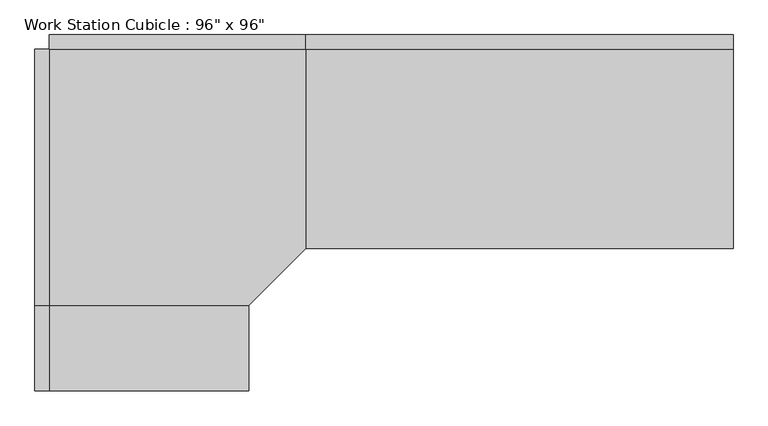
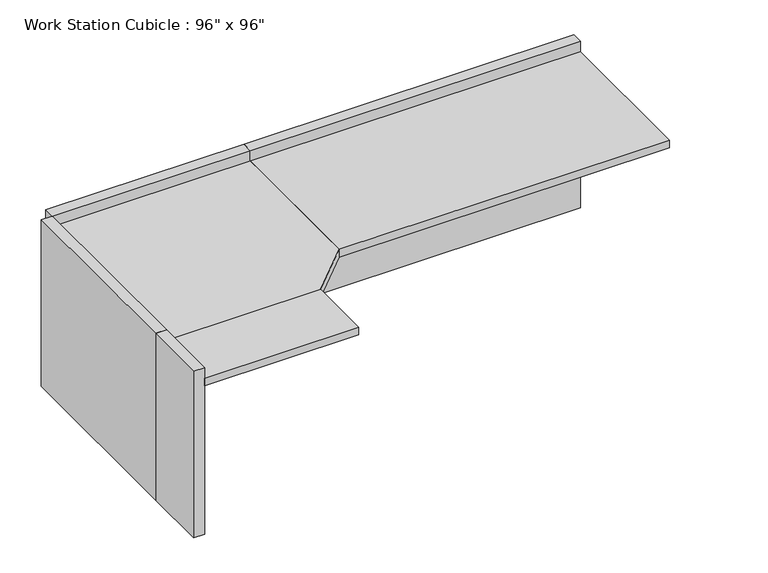
"""IFC4 building model written with IfcOpenShell, lengths in millimetres: furniture geometry."""

from ifc_helpers import new_model, si_unit, frame, origin, origin_with_axes, place, context, project, spatial, polyline, outline, extrude, source, transform, mapped, element, save


def furniture_823e54a9(model_context):
    return source(origin(), model_context, "Body", "SweptSolid", [
        extrude(outline(polyline([(-80.9317522, -545.8230076), (833.4682478, -545.8230076), (833.4682478, -1257.0230076), (630.2682478, -1460.2230076), (-80.9317522, -1460.2230076), (-80.9317522, -545.8230076)])), frame((0.0, 0.0, 723.9), z_axis=(0.0, 0.0, 1.0), x_axis=(1.0, 0.0, 0.0)), (0.0, 0.0, 1.0), 38.1),
        extrude(outline(polyline([(630.2682478, -1765.0230076), (-80.9317522, -1765.0230076), (-80.9317522, -1460.2230076), (630.2682478, -1460.2230076), (630.2682478, -1765.0230076)])), frame((0.0, 0.0, 723.9), z_axis=(0.0, 0.0, 1.0), x_axis=(1.0, 0.0, 0.0)), (0.0, 0.0, 1.0), 38.1),
        extrude(outline(polyline([(2357.4682478, -1257.0230076), (833.4682478, -1257.0230076), (833.4682478, -545.8230076), (2357.4682478, -545.8230076), (2357.4682478, -1257.0230076)])), frame((0.0, 0.0, 723.9), z_axis=(0.0, 0.0, 1.0), x_axis=(1.0, 0.0, 0.0)), (0.0, 0.0, 1.0), 38.1),
        extrude(outline(polyline([(2357.4682478, -545.8230076), (833.4682478, -545.8230076), (833.4682478, -495.0230076), (2357.4682478, -495.0230076), (2357.4682478, -545.8230076)])), origin_with_axes(), (0.0, 0.0, 1.0), 812.8),
        extrude(outline(polyline([(833.4682478, -545.8230076), (-80.9317522, -545.8230076), (-80.9317522, -495.0230076), (833.4682478, -495.0230076), (833.4682478, -545.8230076)])), origin_with_axes(), (0.0, 0.0, 1.0), 812.8),
        extrude(outline(polyline([(-80.9317522, -1460.2230076), (-131.7317522, -1460.2230076), (-131.7317522, -545.8230076), (-80.9317522, -545.8230076), (-80.9317522, -1460.2230076)])), origin_with_axes(), (0.0, 0.0, 1.0), 812.8),
        extrude(outline(polyline([(-80.9317522, -1765.0230076), (-131.7317522, -1765.0230076), (-131.7317522, -1460.2230076), (-80.9317522, -1460.2230076), (-80.9317522, -1765.0230076)])), origin_with_axes(), (0.0, 0.0, 1.0), 812.8),
    ])


if __name__ == "__main__":
    model = new_model("IFC4")
    model_context = context("Model", 3, world=origin())
    ifc_project = project(units=[si_unit("LENGTHUNIT", "METRE", prefix="MILLI")], contexts=[model_context])
    site = spatial("IfcSite", under=ifc_project)
    building = spatial("IfcBuilding", under=site)
    placement = place(None, origin())
    furniture_shape = furniture_823e54a9(model_context)
    element("IfcFurniture", 1, ObjectType="Work Station Cubicle : 96\" x 96\"", at=placement, inside=building, context=model_context, shape_type="MappedRepresentation", body=[
        mapped(furniture_shape, transform((0.0, 0.0, 0.0), x_axis=(1.0, 0.0, 0.0), y_axis=(0.0, 1.0, 0.0), z_axis=(0.0, 0.0, 1.0))),
    ])
    save(model, "model.ifc")

# Revit data of these elements
# Type "Work Station Cubicle : 96\" x 96\""
#   Assembly Code = "E2020"
#   Desktop Height = 2' - 6"
#   Desktop1 Width = 2' - 4"
#   Desktop2 Width = 2' - 4"
#   Panel Height = 2' - 8"
#   Panel1 Length = 1' - 0"
#   Panel2 Length = 5' - 0"
#   Cube Panel Material = Textile - Light Gray
#   Work Top Material = Laminate, Ivory, Matte
#   Default Elevation = 0
# Element 1 (IfcFurniture, "Work Station Cubicle : 96\" x 96\"")
#   Materials on its faces: "Textile - Light Gray", "Laminate, Ivory, Matte"
# Materials
#   "Textile - Light Gray": class "Fabric", colour RGB 204 204 204, transparency 0
#   "Laminate, Ivory, Matte": class "Plastic", colour RGB 247 247 239, transparency 0, Description = "Plastic Laminate - Ivory, Matte", Cost = 0
